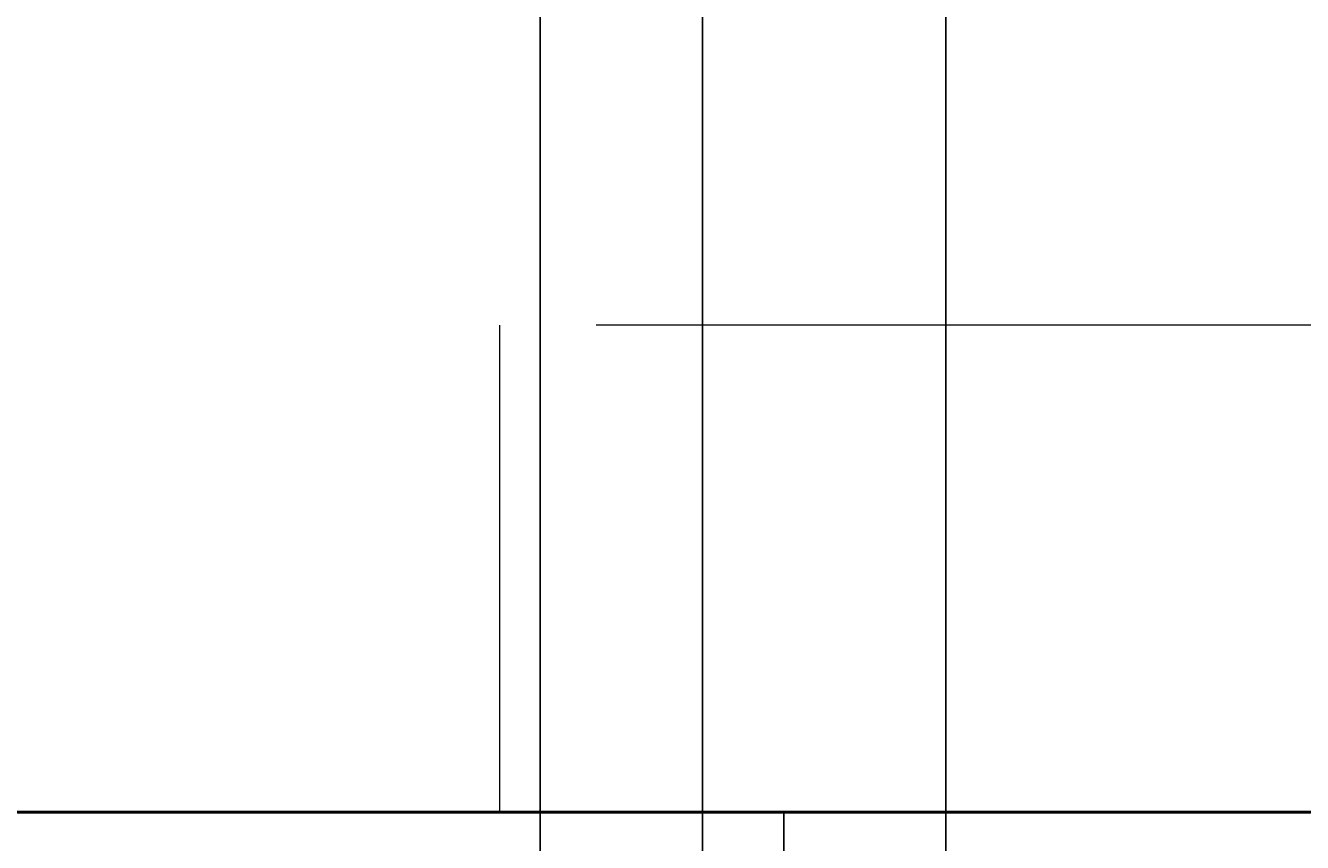
# Model space of a CAD drawing. Units: inches. Extents: x 37 to 824, y -700 to 234.
# Tile 58 of 77: x 193 to 225, y 190 to 210. Entities that reach past the tile are written whole.
import ezdxf

# ---------------------------------------------------------------- set-up
doc = ezdxf.new("R2010")
doc.units = ezdxf.units.IN
doc.header["$MEASUREMENT"] = 0
doc.linetypes.add('DASHED', pattern=[19.05, 12.7, -6.35])
for name, color, linetype, lineweight in [('A-ANNO-DIMS', 2, 'Continuous', 18), ('A-GLAZ', 4, 'Continuous', 25), ('A-ROOF-OVHD', 1, 'DASHED', 18), ('A-WALL', 2, 'Continuous', 50)]:
    doc.layers.add(name, color=color, linetype=linetype, lineweight=lineweight)
doc.styles.get("Standard").update_dxf_attribs({"font": 'arial.ttf'})
doc.dimstyles.get("Standard").update_dxf_attribs({"dimtxt": 0.18, "dimasz": 0.18, "dimexe": 0.18, "dimexo": 0.0625, "dimgap": 0.09, "dimtad": 0, "dimtih": 1, "dimtoh": 1, "dimdec": 1, "dimzin": 0, "dimdsep": 46, "dimlunit": 4, "dimtxsty": 'Standard', "dimcen": 0.09, "dimadec": 0, "dimazin": 0, "dimtfac": 1, "dimtdec": 1, "dimtofl": 0, "dimtmove": 0, "dimatfit": 3, "dimfxl": 1, "dimtolj": 1, "dimtzin": 0, "dimarcsym": 0})

# ---------------------------------------------------------------- blocks, each defined once
blk = doc.blocks.new('WIN-900')
for p, q in [((38, 9), (38, 0)), ((40, 9), (40, 0))]:
    blk.add_line(p, q)
blk = doc.blocks.new('*D44')
at = {"layer": 'A-ANNO-DIMS', "color": 0, "lineweight": -2, "ltscale": 0.5, "transparency": 16777216}
for p, q in [((161.077, 191.153), (161.077, 234.17)), ((210.077, 191.153), (210.077, 234.17)), ((161.257, 233.99), (185.244, 233.99)), ((209.897, 233.99), (185.91, 233.99))]:
    blk.add_line(p, q, dxfattribs=at)
at = {"layer": 'A-ANNO-DIMS', "color": 0, "ltscale": 0.5, "transparency": 16777216}
for points in [[(161.257, 234.02), (161.257, 233.96), (161.077, 233.99)], [(209.897, 234.02), (209.897, 233.96), (210.077, 233.99)]]:
    blk.add_solid(points, dxfattribs=at)
at = {"layer": 'Defpoints', "color": 0, "ltscale": 0.5, "transparency": 16777216}
for p in [(210.077, 233.99), (161.077, 191.09), (210.077, 191.09)]:
    blk.add_point(p, dxfattribs=at)
at = {"layer": 'A-ANNO-DIMS', "color": 0, "ltscale": 0.5, "transparency": 16777216, "insert": (185.577, 233.99), "char_height": 0.18, "attachment_point": 5}
blk.add_mtext('\\A1;4\'-1"', dxfattribs=at)
blk = doc.blocks.new('*D45')
at = {"layer": 'A-ANNO-DIMS', "color": 0, "lineweight": -2, "ltscale": 0.5, "transparency": 16777216}
for p, q in [((210.077, 191.153), (210.077, 234.17)), ((250.077, 191.153), (250.077, 234.17)), ((210.257, 233.99), (229.748, 233.99)), ((249.897, 233.99), (230.406, 233.99))]:
    blk.add_line(p, q, dxfattribs=at)
at = {"layer": 'A-ANNO-DIMS', "color": 0, "ltscale": 0.5, "transparency": 16777216}
for points in [[(210.257, 234.02), (210.257, 233.96), (210.077, 233.99)], [(249.897, 234.02), (249.897, 233.96), (250.077, 233.99)]]:
    blk.add_solid(points, dxfattribs=at)
at = {"layer": 'Defpoints', "color": 0, "ltscale": 0.5, "transparency": 16777216}
for p in [(250.077, 233.99), (210.077, 191.09), (250.077, 191.09)]:
    blk.add_point(p, dxfattribs=at)
at = {"layer": 'A-ANNO-DIMS', "color": 0, "ltscale": 0.5, "transparency": 16777216, "insert": (230.077, 233.99), "char_height": 0.18, "attachment_point": 5}
blk.add_mtext('\\A1;3\'-4"', dxfattribs=at)
blk = doc.blocks.new('*D63')
at = {"layer": 'A-ANNO-DIMS', "color": 0, "lineweight": -2, "ltscale": 0.5, "transparency": 16777216}
for p, q in [((161.077, 191.153), (161.077, 234.17)), ((428.077, 191.153), (428.077, 234.17)), ((161.257, 233.99), (294.176, 233.99)), ((427.897, 233.99), (294.978, 233.99))]:
    blk.add_line(p, q, dxfattribs=at)
at = {"layer": 'A-ANNO-DIMS', "color": 0, "ltscale": 0.5, "transparency": 16777216}
for points in [[(161.257, 234.02), (161.257, 233.96), (161.077, 233.99)], [(427.897, 234.02), (427.897, 233.96), (428.077, 233.99)]]:
    blk.add_solid(points, dxfattribs=at)
at = {"layer": 'Defpoints', "color": 0, "ltscale": 0.5, "transparency": 16777216}
for p in [(428.077, 233.99), (161.077, 191.09), (428.077, 191.09)]:
    blk.add_point(p, dxfattribs=at)
at = {"layer": 'A-ANNO-DIMS', "color": 0, "ltscale": 0.5, "transparency": 16777216, "insert": (294.577, 233.99), "char_height": 0.18, "attachment_point": 5}
blk.add_mtext('\\A1;22\'-3"', dxfattribs=at)
blk = doc.blocks.new('*D72')
at = {"layer": 'A-ANNO-DIMS', "color": 0, "lineweight": -2, "ltscale": 0.5, "transparency": 16777216}
for p, q in [((170.077, 84.153), (170.077, 234.17)), ((250.19, 84.153), (250.19, 234.17)), ((170.257, 233.99), (209.804, 233.99)), ((250.01, 233.99), (210.463, 233.99))]:
    blk.add_line(p, q, dxfattribs=at)
at = {"layer": 'A-ANNO-DIMS', "color": 0, "ltscale": 0.5, "transparency": 16777216}
for points in [[(170.257, 234.02), (170.257, 233.96), (170.077, 233.99)], [(250.01, 234.02), (250.01, 233.96), (250.19, 233.99)]]:
    blk.add_solid(points, dxfattribs=at)
at = {"layer": 'Defpoints', "color": 0, "ltscale": 0.5, "transparency": 16777216}
for p in [(250.19, 233.99), (170.077, 84.09), (250.19, 84.09)]:
    blk.add_point(p, dxfattribs=at)
at = {"layer": 'A-ANNO-DIMS', "color": 0, "ltscale": 0.5, "transparency": 16777216, "insert": (210.133, 233.99), "char_height": 0.18, "attachment_point": 5}
blk.add_mtext('\\A1;6\'-8"', dxfattribs=at)
blk = doc.blocks.new('*D84')
at = {"layer": 'A-ANNO-DIMS', "color": 0, "lineweight": -2, "ltscale": 0.5, "transparency": 16777216}
for p, q in [((170.077, -265.847), (170.077, 234.17)), ((210.077, -265.847), (210.077, 234.17)), ((170.257, 233.99), (189.748, 233.99)), ((209.897, 233.99), (190.406, 233.99))]:
    blk.add_line(p, q, dxfattribs=at)
at = {"layer": 'A-ANNO-DIMS', "color": 0, "ltscale": 0.5, "transparency": 16777216}
for points in [[(170.257, 234.02), (170.257, 233.96), (170.077, 233.99)], [(209.897, 234.02), (209.897, 233.96), (210.077, 233.99)]]:
    blk.add_solid(points, dxfattribs=at)
at = {"layer": 'Defpoints', "color": 0, "ltscale": 0.5, "transparency": 16777216}
for p in [(210.077, 233.99), (170.077, -265.91), (210.077, -265.91)]:
    blk.add_point(p, dxfattribs=at)
at = {"layer": 'A-ANNO-DIMS', "color": 0, "ltscale": 0.5, "transparency": 16777216, "insert": (190.077, 233.99), "char_height": 0.18, "attachment_point": 5}
blk.add_mtext('\\A1;3\'-4"', dxfattribs=at)
blk = doc.blocks.new('*D85')
at = {"layer": 'A-ANNO-DIMS', "color": 0, "lineweight": -2, "ltscale": 0.5, "transparency": 16777216}
for p, q in [((170.077, -356.847), (170.077, 234.17)), ((206.077, -356.847), (206.077, 234.17)), ((170.257, 233.99), (187.748, 233.99)), ((205.897, 233.99), (188.406, 233.99))]:
    blk.add_line(p, q, dxfattribs=at)
at = {"layer": 'A-ANNO-DIMS', "color": 0, "ltscale": 0.5, "transparency": 16777216}
for points in [[(170.257, 234.02), (170.257, 233.96), (170.077, 233.99)], [(205.897, 234.02), (205.897, 233.96), (206.077, 233.99)]]:
    blk.add_solid(points, dxfattribs=at)
at = {"layer": 'Defpoints', "color": 0, "ltscale": 0.5, "transparency": 16777216}
for p in [(206.077, 233.99), (170.077, -356.91), (206.077, -356.91)]:
    blk.add_point(p, dxfattribs=at)
at = {"layer": 'A-ANNO-DIMS', "color": 0, "ltscale": 0.5, "transparency": 16777216, "insert": (188.077, 233.99), "char_height": 0.18, "attachment_point": 5}
blk.add_mtext('\\A1;3\'-0"', dxfattribs=at)
blk = doc.blocks.new('*D86')
at = {"layer": 'A-ANNO-DIMS', "color": 0, "lineweight": -2, "ltscale": 0.5, "transparency": 16777216}
for p, q in [((206.077, -356.847), (206.077, 234.17)), ((216.077, -356.847), (216.077, 234.17)), ((206.257, 233.99), (210.678, 233.99)), ((215.897, 233.99), (211.476, 233.99))]:
    blk.add_line(p, q, dxfattribs=at)
at = {"layer": 'A-ANNO-DIMS', "color": 0, "ltscale": 0.5, "transparency": 16777216}
for points in [[(206.257, 234.02), (206.257, 233.96), (206.077, 233.99)], [(215.897, 234.02), (215.897, 233.96), (216.077, 233.99)]]:
    blk.add_solid(points, dxfattribs=at)
at = {"layer": 'Defpoints', "color": 0, "ltscale": 0.5, "transparency": 16777216}
for p in [(216.077, 233.99), (206.077, -356.91), (216.077, -356.91)]:
    blk.add_point(p, dxfattribs=at)
at = {"layer": 'A-ANNO-DIMS', "color": 0, "ltscale": 0.5, "transparency": 16777216, "insert": (211.077, 233.99), "char_height": 0.18, "attachment_point": 5}
blk.add_mtext('\\A1;0\'-10"', dxfattribs=at)
blk = doc.blocks.new('*D87')
at = {"layer": 'A-ANNO-DIMS', "color": 0, "lineweight": -2, "ltscale": 0.5, "transparency": 16777216}
for p, q in [((216.077, -356.847), (216.077, 234.17)), ((296.077, -356.847), (296.077, 234.17)), ((216.257, 233.99), (255.747, 233.99)), ((295.897, 233.99), (256.407, 233.99))]:
    blk.add_line(p, q, dxfattribs=at)
at = {"layer": 'A-ANNO-DIMS', "color": 0, "ltscale": 0.5, "transparency": 16777216}
for points in [[(216.257, 234.02), (216.257, 233.96), (216.077, 233.99)], [(295.897, 234.02), (295.897, 233.96), (296.077, 233.99)]]:
    blk.add_solid(points, dxfattribs=at)
at = {"layer": 'Defpoints', "color": 0, "ltscale": 0.5, "transparency": 16777216}
for p in [(296.077, 233.99), (216.077, -356.91), (296.077, -356.91)]:
    blk.add_point(p, dxfattribs=at)
at = {"layer": 'A-ANNO-DIMS', "color": 0, "ltscale": 0.5, "transparency": 16777216, "insert": (256.077, 233.99), "char_height": 0.18, "attachment_point": 5}
blk.add_mtext('\\A1;6\'-8"', dxfattribs=at)

msp = doc.modelspace()

# ---------------------------------------------------------------- linework, layer by layer
at = {"layer": 'A-ROOF-OVHD', "ltscale": 1.5}
for p, q in [((205.077, 191.09), (205.077, 203.09)), ((255.077, 203.09), (205.077, 203.09)), ((210.077, 191.09), (205.077, 191.09))]:
    msp.add_line(p, q, dxfattribs=at)
at = {"layer": 'A-WALL'}
msp.add_line((161.077, 191.09), (299.077, 191.09), dxfattribs=at)

# ---------------------------------------------------------------- block references
at = {"layer": 'A-GLAZ', "rotation": 180}
msp.add_blockref('WIN-900', (250.077, 191.091), dxfattribs=at)

# ---------------------------------------------------------------- dimensions: what is measured, and where the dimension line sits
at = {"layer": 'A-ANNO-DIMS', "ltscale": 0.5}
for base, p1, p2, picture, middle in [((210.077, 233.99), (161.077, 191.09), (210.077, 191.09), '*D44', (185.577, 233.99)), ((428.077, 233.99), (161.077, 191.09), (428.077, 191.09), '*D63', (294.577, 233.99)), ((250.19, 233.99), (170.077, 84.09), (250.19, 84.09), '*D72', (210.133, 233.99)), ((210.077, 233.99), (170.077, -265.91), (210.077, -265.91), '*D84', (190.077, 233.99)), ((206.077, 233.99), (170.077, -356.91), (206.077, -356.91), '*D85', (188.077, 233.99)), ((216.077, 233.99), (206.077, -356.91), (216.077, -356.91), '*D86', (211.077, 233.99)), ((250.077, 233.99), (210.077, 191.09), (250.077, 191.09), '*D45', (230.077, 233.99)), ((296.077, 233.99), (216.077, -356.91), (296.077, -356.91), '*D87', (256.077, 233.99))]:
    dim = msp.add_linear_dim(base=base, p1=p1, p2=p2, dimstyle='Standard', override={"dimdec": 1, "dimlfac": 1, "dimrnd": 0, "dimzin": 1, "dimdsep": 46, "dimlunit": 4, "dimfrac": 2}, dxfattribs=at)
    dim.commit()
    dim.dimension.update_dxf_attribs({"geometry": picture, "text_midpoint": middle})

doc.saveas('drawing.dxf')
